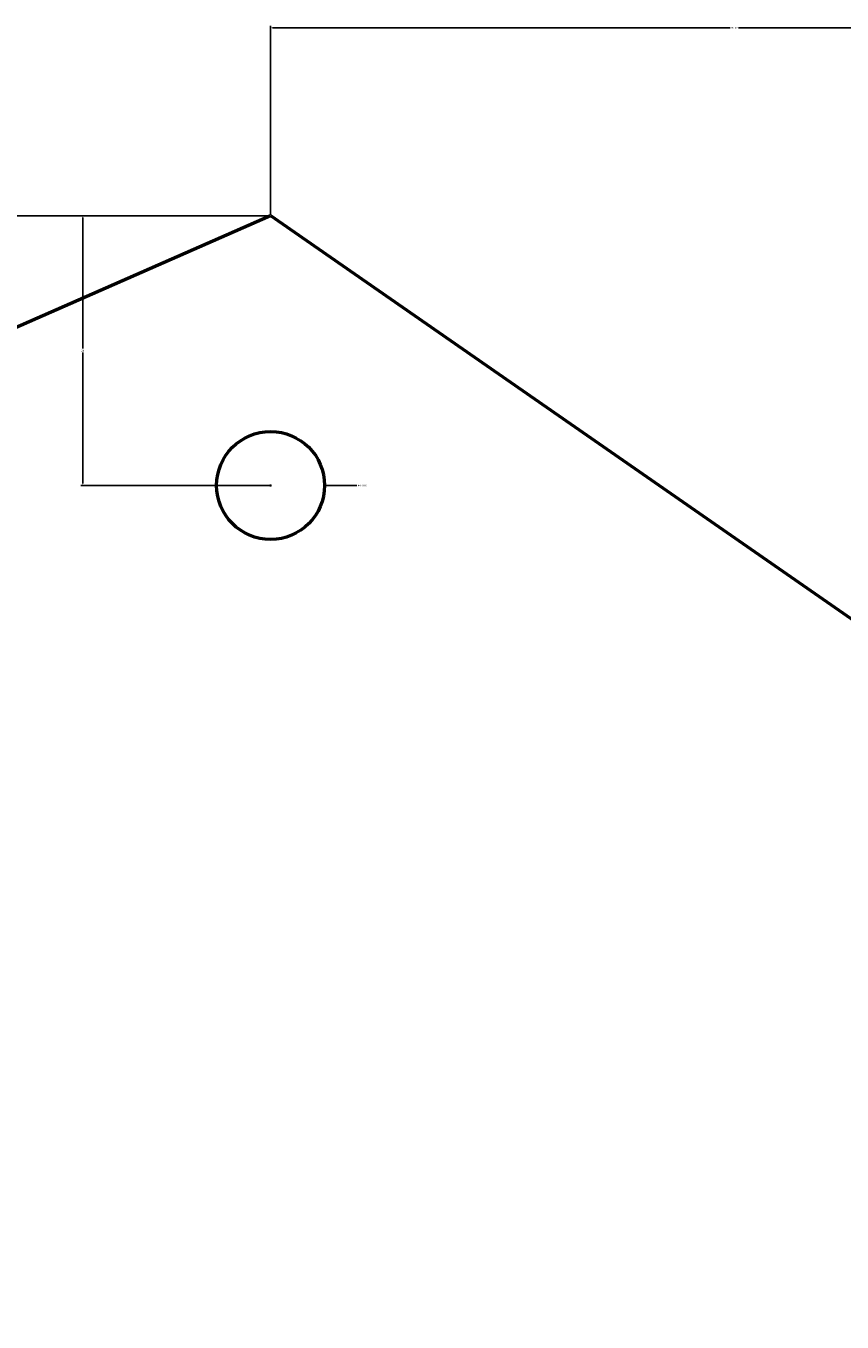
# Model space of a CAD drawing. Units: inches. Extents: x 457 to 775, y 319 to 541.
# Tile 11 of 12: x 623 to 699, y 421 to 541. Entities that reach past the tile are written whole.
import ezdxf

# ---------------------------------------------------------------- set-up
doc = ezdxf.new("R2010")
doc.units = ezdxf.units.IN
doc.header["$MEASUREMENT"] = 0
doc.layers.add('M-DIMS', color=2, linetype='Continuous', lineweight=18)
doc.layers.add('M-OUTL', color=7, linetype='Continuous', lineweight=50)
doc.styles.get("Standard").update_dxf_attribs({"font": 'arial.ttf'})
doc.dimstyles.get("Standard").update_dxf_attribs({"dimtxt": 0.18, "dimasz": 0.18, "dimexe": 0.18, "dimexo": 0.0625, "dimgap": 0.09, "dimtad": 0, "dimtih": 1, "dimtoh": 1, "dimdec": 4, "dimzin": 0, "dimdsep": 46, "dimtxsty": 'Standard', "dimcen": 0.09, "dimadec": 0, "dimazin": 0, "dimtfac": 1, "dimtdec": 4, "dimtofl": 0, "dimtmove": 0, "dimatfit": 3, "dimfxl": 1, "dimtolj": 1, "dimtzin": 0, "dimarcsym": 0})

# ---------------------------------------------------------------- blocks, each defined once
blk = doc.blocks.new('MOUNT-HOLE-D10')
blk.add_circle((5, 5), 5)
blk = doc.blocks.new('*D3')
at = {"layer": 'Defpoints', "color": 0, "transparency": 16777216}
for p in [(456.91, 523.21), (646, 523.21), (474.31, 336.7)]:
    blk.add_point(p, dxfattribs=at)
at = {"layer": 'M-DIMS', "color": 0, "lineweight": -2, "transparency": 16777216}
for p, q in [((645.94, 523.21), (456.73, 523.21)), ((456.91, 523.03), (456.91, 430.14)), ((456.91, 336.88), (456.91, 429.77)), ((474.24, 336.7), (456.73, 336.7))]:
    blk.add_line(p, q, dxfattribs=at)
at = {"layer": 'M-DIMS', "color": 0, "transparency": 16777216}
for points in [[(456.88, 523.03), (456.94, 523.03), (456.91, 523.21)], [(456.88, 336.88), (456.94, 336.88), (456.91, 336.7)]]:
    blk.add_solid(points, dxfattribs=at)
at = {"layer": 'M-DIMS', "color": 0, "transparency": 16777216, "insert": (456.91, 429.95), "char_height": 0.18, "attachment_point": 5}
blk.add_mtext('\\A1;186.5', dxfattribs=at)
blk = doc.blocks.new('*D4')
at = {"layer": 'Defpoints', "color": 0, "transparency": 16777216}
for p in [(731.93, 540.61), (646, 523.21), (731.93, 433.2)]:
    blk.add_point(p, dxfattribs=at)
at = {"layer": 'M-DIMS', "color": 0, "lineweight": -2, "transparency": 16777216}
for p, q in [((646, 523.28), (646, 540.79)), ((646.18, 540.61), (688.57, 540.61)), ((731.75, 540.61), (689.36, 540.61)), ((731.93, 433.26), (731.93, 540.79))]:
    blk.add_line(p, q, dxfattribs=at)
at = {"layer": 'M-DIMS', "color": 0, "transparency": 16777216}
for points in [[(646.18, 540.64), (646.18, 540.58), (646, 540.61)], [(731.75, 540.64), (731.75, 540.58), (731.93, 540.61)]]:
    blk.add_solid(points, dxfattribs=at)
at = {"layer": 'M-DIMS', "color": 0, "transparency": 16777216, "insert": (688.97, 540.61), "char_height": 0.18, "attachment_point": 5}
blk.add_mtext('\\A1;85.93', dxfattribs=at)
blk = doc.blocks.new('*D8')
at = {"layer": 'Defpoints', "color": 0, "transparency": 16777216}
for p in [(628.6, 523.21), (646, 523.21), (646, 498.21)]:
    blk.add_point(p, dxfattribs=at)
at = {"layer": 'M-DIMS', "color": 0, "lineweight": -2, "transparency": 16777216}
for p, q in [((645.94, 523.21), (628.42, 523.21)), ((628.6, 523.03), (628.6, 510.89)), ((628.6, 498.39), (628.6, 510.53)), ((645.94, 498.21), (628.42, 498.21))]:
    blk.add_line(p, q, dxfattribs=at)
at = {"layer": 'M-DIMS', "color": 0, "transparency": 16777216}
for points in [[(628.57, 523.03), (628.63, 523.03), (628.6, 523.21)], [(628.57, 498.39), (628.63, 498.39), (628.6, 498.21)]]:
    blk.add_solid(points, dxfattribs=at)
at = {"layer": 'M-DIMS', "color": 0, "transparency": 16777216, "insert": (628.6, 510.71), "char_height": 0.18, "attachment_point": 5}
blk.add_mtext('\\A1;25', dxfattribs=at)
blk = doc.blocks.new('*D23')
at = {"layer": 'Defpoints', "color": 0, "transparency": 16777216}
for p in [(641, 498.21), (651, 498.21)]:
    blk.add_point(p, dxfattribs=at)
at = {"layer": 'M-DIMS', "color": 0, "lineweight": -2, "transparency": 16777216}
for p, q in [((645.91, 498.21), (646.09, 498.21)), ((646, 498.12), (646, 498.3)), ((654, 498.21), (651.18, 498.21))]:
    blk.add_line(p, q, dxfattribs=at)
at = {"layer": 'M-DIMS', "color": 0, "transparency": 16777216}
blk.add_solid([(651.18, 498.24), (651.18, 498.18), (651, 498.21)], dxfattribs=at)
at = {"layer": 'M-DIMS', "color": 0, "transparency": 16777216, "insert": (654.51, 498.21), "char_height": 0.18, "attachment_point": 5}
blk.add_mtext('\\A1;4X ∅10', dxfattribs=at)

msp = doc.modelspace()

# ---------------------------------------------------------------- linework, layer by layer
at = {"layer": 'M-OUTL'}
for p, q in [((474.306, 448.059), (646.001, 523.213)), ((646.001, 523.213), (744.409, 454.859))]:
    msp.add_line(p, q, dxfattribs=at)

# ---------------------------------------------------------------- block references
msp.add_blockref('MOUNT-HOLE-D10', (641.001, 493.213), dxfattribs=at)

# ---------------------------------------------------------------- dimensions: what is measured, and where the dimension line sits
at = {"layer": 'M-DIMS'}
dim = msp.add_linear_dim(base=(731.931, 540.613), p1=(646.001, 523.213), p2=(731.931, 433.196), dimstyle='Standard', override={"dimdec": 2, "dimlfac": 1, "dimrnd": 0, "dimzin": 0, "dimdsep": 46, "dimlunit": 2}, dxfattribs=at)
dim.commit()
dim.dimension.update_dxf_attribs({"geometry": '*D4', "text_midpoint": (688.966, 540.613)})
for base, p1, override, picture, middle in [((456.906, 523.213), (474.306, 336.696), {"dimdec": 1, "dimlfac": 1, "dimrnd": 0, "dimzin": 0, "dimdsep": 46, "dimlunit": 2}, '*D3', (456.906, 429.954)), ((628.601, 523.213), (646.001, 498.213), {"dimdec": 0, "dimlfac": 1, "dimrnd": 0, "dimzin": 0, "dimdsep": 46, "dimlunit": 2}, '*D8', (628.601, 510.713))]:
    dim = msp.add_linear_dim(base=base, p1=p1, p2=(646.001, 523.213), angle=90, dimstyle='Standard', override=override, dxfattribs=at)
    dim.commit()
    dim.dimension.update_dxf_attribs({"geometry": picture, "text_midpoint": middle})
dim = msp.add_diameter_dim_2p(p1=(641.001, 498.213), p2=(651.001, 498.213), text='4X <>', dimstyle='Standard', override={"dimdec": 0, "dimlfac": 1, "dimrnd": 0, "dimzin": 0, "dimdsep": 46, "dimlunit": 2}, dxfattribs=at)
dim.commit()
dim.dimension.update_dxf_attribs({"geometry": '*D23', "text_midpoint": (654.001, 498.213), "dimtype": 163})

doc.saveas('drawing.dxf')
